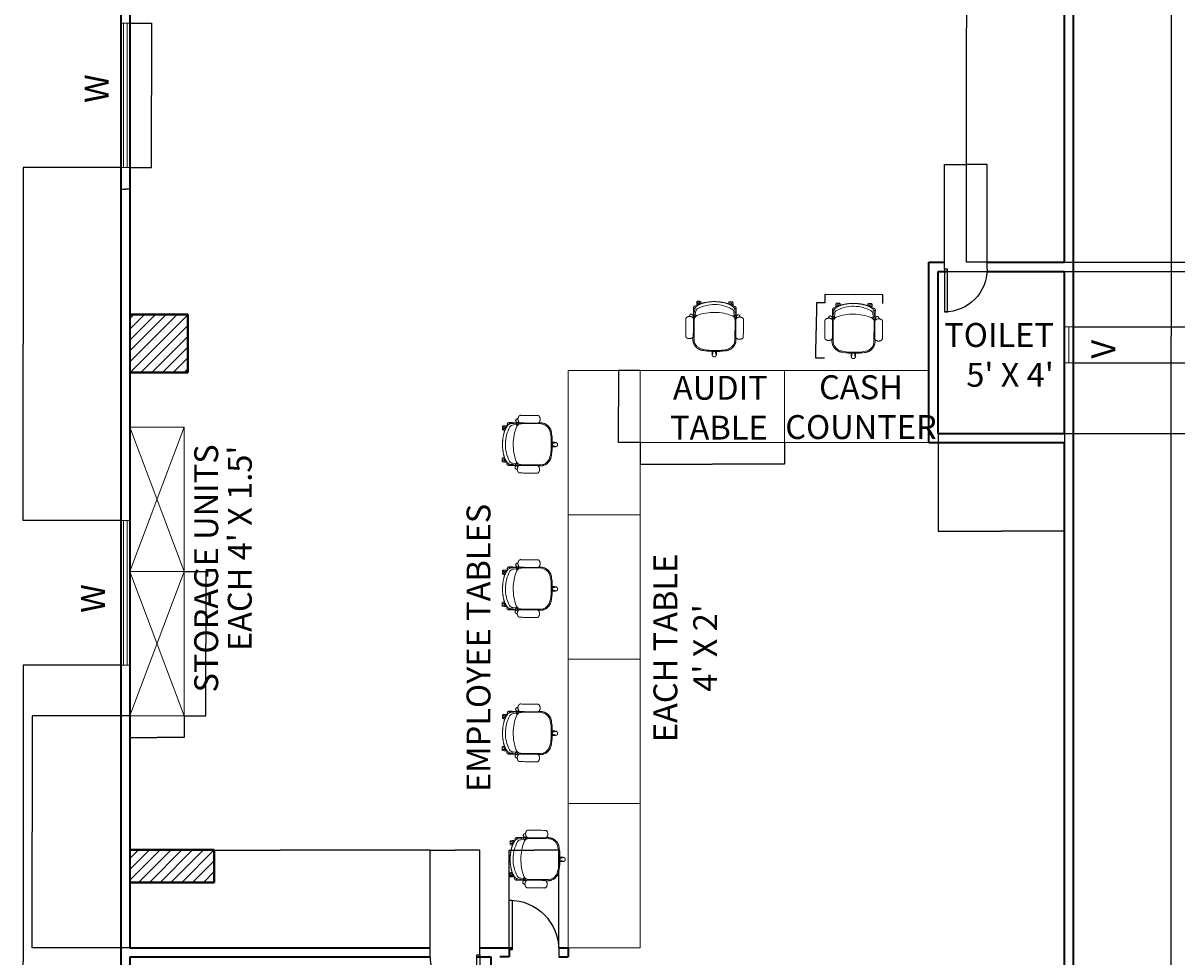
# Model space of a CAD drawing. Units: millimetres. Extents: x -5297 to 19051, y -14478 to 4427.
# Tile 2 of 4: x 1293 to 10888, y -10580 to -2816. Entities that reach past the tile are written whole.
import ezdxf

# ---------------------------------------------------------------- set-up
doc = ezdxf.new("R2010")
doc.units = ezdxf.units.MM
for name, color, linetype, lineweight in [('A-ANNO-DIMS', 2, 'Continuous', 18), ('A-ANNO-TEXT', 7, 'Continuous', 18), ('A-AREA-IDEN', 7, 'Continuous', 25), ('A-COLS', 7, 'Continuous', 40), ('A-COLS-PATT', 252, 'Continuous', 13), ('A-DOOR', 3, 'Continuous', 25), ('A-FLOR-CASE', 9, 'Continuous', 20), ('A-FURN', 8, 'Continuous', 18), ('A-GLAZ', 4, 'Continuous', 18), ('A-WALL', 7, 'Continuous', 35)]:
    doc.layers.add(name, color=color, linetype=linetype, lineweight=lineweight)
doc.styles.get("Standard").update_dxf_attribs({"font": 'arial.ttf'})
doc.dimstyles.get("Standard").update_dxf_attribs({"dimtxt": 0.18, "dimasz": 0.18, "dimexe": 0.18, "dimexo": 0.0625, "dimgap": 0.09, "dimtad": 0, "dimtih": 1, "dimtoh": 1, "dimdec": 4, "dimzin": 0, "dimdsep": 46, "dimtxsty": 'Standard', "dimcen": 0.09, "dimadec": 0, "dimazin": 0, "dimtfac": 1, "dimtdec": 4, "dimtofl": 0, "dimtmove": 0, "dimatfit": 3, "dimfxl": 1, "dimtolj": 1, "dimtzin": 0, "dimarcsym": 0})

# ---------------------------------------------------------------- blocks, each defined once
blk = doc.blocks.new('*U2')
for p, q in [((-700, 0), (-700, -100)), ((0, 0), (0, -100))]:
    blk.add_line(p, q)
blk.add_lwpolyline([(0, 0), (0, 700), (-43.75, 700), (-43.75, 0)], close=True)
blk.add_arc((0, 0), 700, 90, 180)
blk = doc.blocks.new('*U3')
for p, q in [((0, 0), (0, 100)), ((700, 0), (700, 100))]:
    blk.add_line(p, q)
blk.add_lwpolyline([(0, 0), (0, -700), (43.75, -700), (43.75, 0)], close=True)
blk.add_arc((0, 0), 700, 270, 0)
blk = doc.blocks.new('*U4')
for p, q in [((-600, 0), (-600, 100)), ((0, 0), (0, 100))]:
    blk.add_line(p, q)
blk.add_lwpolyline([(0, 0), (0, -600), (-43.75, -600), (-43.75, 0)], close=True)
blk.add_arc((0, 0), 600, 180, 270)
blk = doc.blocks.new('fdss')
at = {"color": 0}
for p, q in [((426, 240), (196, 239)), ((470, 236), (480, 226)), ((480, 225), (479, 223)), ((482, 204), (480, 210)), ((484, 228), (520, 224)), ((617, 196), (646, 196)), ((618, 179), (646, 179)), ((647, 195), (647, 179)), ((426, -240), (196, -239)), ((470, -236), (480, -226)), ((480, -225), (479, -223)), ((482, -204), (480, -210)), ((484, -228), (520, -224)), ((617, -196), (646, -196)), ((618, -179), (646, -179)), ((647, -195), (647, -179))]:
    blk.add_line(p, q, dxfattribs=at)
for points in [[(505, 245), (520, 247), (546, 249), (551, 249)], [(566, 236), (554, 235), (512, 240)], [(33, 21), (34, 20), (36, 19), (37, 18), (37, 18), (39, 18)], [(39, 18), (41, 17), (43, 17), (46, 16), (47, 16), (50, 16), (53, 16), (55, 16), (57, 16), (60, 16), (63, 16)], [(75, -28), (75, 0), (75, 28)], [(33, -21), (34, -20), (36, -19), (37, -18), (37, -18), (39, -18)], [(39, -18), (41, -17), (43, -17), (46, -16), (47, -16), (50, -16), (53, -16), (55, -16), (57, -16), (60, -16), (63, -16)], [(505, -245), (520, -247), (546, -249), (551, -249)], [(566, -236), (554, -235), (512, -240)]]:
    blk.add_lwpolyline(points, dxfattribs=at)
at = {"color": 0, "extrusion": (0, 0, -1)}
for centre, major_axis, start_param, end_param in [((445, 42), (-262, 262), 5.459154, 5.874691), ((201, 128), (-79, 79), 5.969012, 7.027382), ((424, 173), (47, 47), -0.751727, 0.301996), ((424, 175), (54.1, 54.1), -0.544214, -0.156468), ((514, 220), (24.9, 24.9), 3.662908, 4.015109), ((484, 224), (3.3, 3.3), 4.243712, 5.205719), ((484, 229), (-1.47, 1.47), 3.927418, 5.578652), ((-41, 3), (553, 91), -0.204201, 0.167634), ((500, 224), (-12.9, 12.9), 5.819354, 6.506047), ((509, 207), (26.9, 26.9), -1.329065, -0.883773), ((521, 177), (-33.1, 33.1), 0.763307, 1.830683), ((550, 228), (14.8, 14.8), -0.735707, 0.161366), ((545, 180), (-39.3, 39.3), 0.935679, 1.762262), ((193, 0), (-296, 296), 1.856147, 2.355859), ((566, 238), (1.31, 1.31), 0.929037, 2.293349), ((563, 238), (-2.9, 2.9), 1.793197, 2.458506), ((597, 186), (15.6, 15.6), -0.947253, 1.474381), ((621, 198), (-1.12, 1.12), 2.396655, 3.926991), ((621, 177), (-1.12, 1.12), 0.785398, 2.315734), ((646, 195), (0.539, 0.539), -0.785398, 0.785398), ((646, 179), (-0.539, 0.539), 2.356195, 3.926991)]:
    blk.add_ellipse(centre, major_axis=major_axis, ratio=1, start_param=start_param, end_param=end_param, dxfattribs=at)
at = {"color": 0}
for centre, major_axis, start_param, end_param in [((445, -42), (262, 262), 2.317561, 2.733098), ((-41, -3), (-553, 91), 2.937392, 3.309227), ((193, 0), (296, 296), 4.99774, 5.497452), ((201, -128), (79, 79), 2.82742, 3.885789), ((424, -173), (-47, 47), 2.389866, 3.443588), ((424, -175), (-54.1, 54.1), 2.597378, 2.985125), ((514, -220), (-24.9, 24.9), 0.521315, 0.873517), ((484, -224), (-3.3, 3.3), 1.102119, 2.064126), ((484, -229), (1.47, 1.47), 0.785825, 2.437059), ((500, -224), (12.9, 12.9), 2.677762, 3.364454), ((509, -207), (-26.9, 26.9), 1.812527, 2.25782), ((521, -177), (33.1, 33.1), 3.9049, 4.972275), ((550, -228), (-14.8, 14.8), 2.405886, 3.302959), ((545, -180), (39.3, 39.3), 4.077272, 4.903855), ((566, -238), (-1.31, 1.31), 4.07063, 5.434941), ((563, -238), (2.9, 2.9), 4.93479, 5.600098), ((597, -186), (15.6, 15.6), 3.765136, 6.18677), ((621, -177), (1.12, 1.12), 3.926991, 5.457327), ((621, -198), (1.12, 1.12), 5.538248, 7.068583), ((646, -179), (0.539, 0.539), 5.497787, 7.068583), ((646, -195), (-0.539, 0.539), 2.356195, 3.926991)]:
    blk.add_ellipse(centre, major_axis=major_axis, ratio=1, start_param=start_param, end_param=end_param, dxfattribs=at)
for points, weights, knots in [([(436, 337), (338, 337), (240, 337), (234, 338), (228, 335), (217, 328), (212, 315), (204, 293), (212, 271), (217, 258), (228, 251), (234, 248), (240, 248)], [1, 1, 1, 0.962754439438, 1, 0.939418827348, 1, 0.934055427035, 1, 0.939418827348, 1, 0.962754439438, 1], [0, 0, 0, 1, 1, 1.54757, 1.54757, 2.247301, 2.247301, 2.977684, 2.977684, 3.677415, 3.677415, 4.224984, 4.224984, 4.224984]), ([(436, 337), (443, 338), (449, 335), (460, 328), (464, 315), (473, 293), (464, 271), (460, 258), (449, 251), (443, 248), (436, 248), (338, 248), (240, 248)], [1, 0.96275443944, 1, 0.939418827348, 1, 0.934055427035, 1, 0.939418827348, 1, 0.96275443944, 1, 1, 1], [0, 0, 0, 0.54757, 0.54757, 1.247301, 1.247301, 1.977684, 1.977684, 2.677415, 2.677415, 3.224984, 3.224984, 4.224984, 4.224984, 4.224984]), ([(468, 296), (480, 296), (489, 288), (493, 285), (494, 280), (496, 274), (494, 268), (488, 255), (474, 254), (463, 254), (452, 253)], [1, 0.943338632687, 1, 0.968267368414, 1, 0.9394851057, 1, 0.864198855487, 1, 1, 1], [0, 0, 0, 0.676489, 0.676489, 1.181677, 1.181677, 1.881021, 1.881021, 2.935502, 2.935502, 3.935502, 3.935502, 3.935502]), ([(227, 252), (219, 252), (211, 252), (156, 255), (115, 218), (74, 180), (72, 125), (63, 75), (63, 25), (63, 13), (62, 0), (63, -13), (63, -25), (63, -75), (72, -125), (74, -180), (115, -218), (156, -255), (211, -252), (219, -252), (227, -252)], [1, 1, 1, 0.920970329426, 1, 0.920970329426, 1, 0.996764637726, 1, 1, 1, 1, 1, 0.996764637726, 1, 0.920970329426, 1, 0.920970329426, 1, 1, 1], [0, 0, 0, 1, 1, 1.800466, 1.800466, 2.600931, 2.600931, 2.761856, 2.761856, 3.761856, 3.761856, 4.761856, 4.761856, 4.922781, 4.922781, 5.723247, 5.723247, 6.523712, 6.523712, 7.523712, 7.523712, 7.523712]), ([(447, 248), (506, 249), (566, 251), (577, 251), (585, 244), (591, 239), (592, 232), (592, 228), (590, 225), (589, 221), (585, 219)], [1, 1, 1, 0.935512434708, 1, 0.918468104225, 1, 0.965843473499, 1, 0.972653000165, 1], [0, 0, 0, 1, 1, 1.722179, 1.722179, 2.535393, 2.535393, 3.059628, 3.059628, 3.528435, 3.528435, 3.528435]), ([(591, 211), (619, 173), (629, 128), (645, 65), (645, 0), (645, -65), (629, -128), (619, -173), (591, -211)], [1, 0.979760898136, 1, 0.992391068779, 1, 0.992391068779, 1, 0.979760898136, 1], [0, 0, 0, 0.403066, 0.403066, 0.649944, 0.649944, 0.896822, 0.896822, 1.299888, 1.299888, 1.299888]), ([(592, 211), (618, 216), (643, 209), (646, 209), (646, 206), (646, 203), (646, 199), (646, 198), (644, 198), (630, 198), (616, 198)], [1, 0.974666881773, 1, 0.783317345499, 1, 1, 1, 0.707106807826, 1, 1, 1], [0, 0, 0, 0.451139, 0.451139, 1.792762, 1.792762, 2.792762, 2.792762, 4.363559, 4.363559, 5.363559, 5.363559, 5.363559]), ([(618, 177), (631, 177), (644, 177), (645, 177), (645, 176), (646, 176), (646, 175), (646, 172), (646, 168), (646, 166), (643, 165), (631, 161), (619, 161)], [1, 1, 1, 0.923879528314, 1, 0.923879528314, 1, 1, 1, 0.783317456604, 1, 0.992237440768, 1], [0, 0, 0, 1, 1, 1.785398, 1.785398, 2.570796, 2.570796, 3.570796, 3.570796, 4.912419, 4.912419, 5.161781, 5.161781, 5.161781]), ([(33, -20), (22, -27), (10, -20), (-1, -13), (0, 0), (-1, 13), (10, 20), (22, 27), (33, 20)], [1, 0.85579821339, 1, 0.85579821339, 1, 0.855798213391, 1, 0.855798213391, 1], [0, 0, 0, 1.087409, 1.087409, 2.174818, 2.174818, 3.262227, 3.262227, 4.349636, 4.349636, 4.349636]), ([(12, 21), (13, 23), (15, 23), (39, 29), (63, 25)], [1, 0.873023611703, 1, 0.980536821249, 1], [0, 0, 0, 1.018856, 1.018856, 1.414094, 1.414094, 1.414094]), ([(12, -21), (13, -23), (15, -23), (39, -29), (63, -25)], [1, 0.873023611717, 1, 0.980536821249, 1], [0, 0, 0, 1.018856, 1.018856, 1.414094, 1.414094, 1.414094]), ([(464, -271), (460, -258), (449, -251), (443, -248), (436, -248), (338, -248), (240, -248), (234, -248), (228, -251), (217, -258), (212, -271), (204, -293), (212, -315), (217, -328), (228, -335), (234, -338), (240, -337), (338, -337), (436, -337)], [1, 0.939418827349, 1, 0.96275443944, 1, 1, 1, 0.962754439438, 1, 0.939418827349, 1, 0.934055427035, 1, 0.939418827348, 1, 0.962754439438, 1, 1, 1], [0, 0, 0, 0.699731, 0.699731, 1.247301, 1.247301, 2.247301, 2.247301, 2.794871, 2.794871, 3.494602, 3.494602, 4.224984, 4.224984, 4.924715, 4.924715, 5.472285, 5.472285, 6.472285, 6.472285, 6.472285]), ([(447, -248), (506, -249), (566, -251), (577, -251), (585, -244), (591, -239), (592, -232), (592, -228), (590, -225), (589, -221), (585, -219)], [1, 1, 1, 0.935512434708, 1, 0.918468104224, 1, 0.965843473499, 1, 0.972653000166, 1], [0, 0, 0, 1, 1, 1.722179, 1.722179, 2.535393, 2.535393, 3.059628, 3.059628, 3.528435, 3.528435, 3.528435]), ([(468, -296), (480, -296), (489, -288), (493, -285), (494, -280), (496, -274), (494, -268), (488, -255), (474, -254), (463, -254), (452, -253)], [1, 0.943338632687, 1, 0.968267368413, 1, 0.9394851057, 1, 0.864198855486, 1, 1, 1], [0, 0, 0, 0.676489, 0.676489, 1.181677, 1.181677, 1.881021, 1.881021, 2.935502, 2.935502, 3.935502, 3.935502, 3.935502]), ([(592, -211), (618, -216), (643, -209), (646, -209), (646, -206), (646, -203), (646, -199), (646, -198), (644, -198), (630, -198), (616, -198)], [1, 0.974666881774, 1, 0.7833173455, 1, 1, 1, 0.707106807832, 1, 1, 1], [0, 0, 0, 0.451139, 0.451139, 1.792762, 1.792762, 2.792762, 2.792762, 4.363559, 4.363559, 5.363559, 5.363559, 5.363559]), ([(618, -177), (631, -177), (644, -177), (645, -177), (645, -176), (646, -176), (646, -175), (646, -172), (646, -168), (646, -166), (643, -165), (631, -161), (619, -161)], [1, 1, 1, 0.923879528318, 1, 0.923879528318, 1, 1, 1, 0.783317456602, 1, 0.992237440768, 1], [0, 0, 0, 1, 1, 1.785398, 1.785398, 2.570796, 2.570796, 3.570796, 3.570796, 4.912419, 4.912419, 5.161781, 5.161781, 5.161781]), ([(464, -271), (473, -293), (464, -315), (460, -328), (449, -335), (443, -338), (436, -337)], [1, 0.934055427035, 1, 0.939418827348, 1, 0.96275443944, 1], [0, 0, 0, 0.730383, 0.730383, 1.430114, 1.430114, 1.977684, 1.977684, 1.977684])]:
    blk.add_rational_spline(points, weights, degree=2, knots=knots, dxfattribs=at)
blk = doc.blocks.new('TABLE-1200x600')
for p, q in [((0, 0), (0, 1200)), ((0, 1200), (600, 1200)), ((600, 1200), (600, 0)), ((600, 0), (0, 0))]:
    blk.add_line(p, q)
blk = doc.blocks.new('WIN-1200')
for p, q in [((0, 1200.9), (76.2, 1200.9)), ((23.1, 1200.9), (23.1, 0.9)), ((53.1, 1200.9), (53.1, 0.9)), ((0, 0), (76.2, 0))]:
    blk.add_line(p, q)
blk = doc.blocks.new('CABINET-1200x450')
for p, q in [((0, 1200), (450, 1200)), ((0, 0), (0, 1200)), ((450, 1200), (0, 0)), ((450, 0), (0, 1200)), ((450, 1200), (450, 0)), ((450, 0), (0, 0))]:
    blk.add_line(p, q)
blk = doc.blocks.new('*D12')
at = {"layer": 'A-ANNO-DIMS', "color": 0, "lineweight": -2, "transparency": 16777216}
for p, q in [((7962.7, -5142.4), (7963.7, -5070.3)), ((7963.8, -5070.5), (8202.4, -5073.6)), ((8443, -5076.6), (8204.5, -5073.6)), ((8442.3, -5148.5), (8443.2, -5076.5))]:
    blk.add_line(p, q, dxfattribs=at)
at = {"layer": 'A-ANNO-DIMS', "color": 0, "transparency": 16777216}
for points in [[(7963.8, -5070.5), (7963.8, -5070.5), (7963.7, -5070.5)], [(8443, -5076.6), (8443, -5076.7), (8443.2, -5076.6)]]:
    blk.add_solid(points, dxfattribs=at)
at = {"layer": 'Defpoints', "color": 0, "transparency": 16777216}
for p in [(8443.2, -5076.6), (7962.7, -5142.4), (8442.3, -5148.6)]:
    blk.add_point(p, dxfattribs=at)
at = {"layer": 'A-ANNO-DIMS', "color": 0, "transparency": 16777216, "insert": (8203.4, -5073.6), "char_height": 0.18, "attachment_point": 5}
blk.add_mtext('\\A1;CHAIR 480 TYP.', dxfattribs=at)
blk = doc.blocks.new('*D13')
at = {"layer": 'A-ANNO-DIMS', "color": 0, "lineweight": -2, "transparency": 16777216}
for p, q in [((7890.8, -5141.7), (7887.9, -5371.2)), ((7962.7, -5142.4), (7890.6, -5141.5)), ((7884.9, -5601), (7887.9, -5371.5)), ((7956.8, -5602.1), (7884.7, -5601.2))]:
    blk.add_line(p, q, dxfattribs=at)
at = {"layer": 'A-ANNO-DIMS', "color": 0, "transparency": 16777216}
for points in [[(7890.8, -5141.7), (7890.8, -5141.7), (7890.8, -5141.5)], [(7884.9, -5601), (7885, -5601), (7884.9, -5601.2)]]:
    blk.add_solid(points, dxfattribs=at)
at = {"layer": 'Defpoints', "color": 0, "transparency": 16777216}
for p in [(7890.8, -5141.5), (7962.7, -5142.4), (7956.9, -5602.1)]:
    blk.add_point(p, dxfattribs=at)
at = {"layer": 'A-ANNO-DIMS', "color": 0, "transparency": 16777216, "insert": (7887.9, -5371.4), "char_height": 0.18, "attachment_point": 5}
blk.add_mtext('\\A1;460 TYP.', dxfattribs=at)
blk = doc.blocks.new('*D14')
at = {"layer": 'A-ANNO-DIMS', "color": 0, "lineweight": -2, "transparency": 16777216}
for p, q in [((6425, -6303.9), (6425, -6484)), ((7625, -6303.9), (7625, -6484)), ((6425.1, -6483.8), (7023.9, -6483.8)), ((7624.8, -6483.8), (7026.1, -6483.8))]:
    blk.add_line(p, q, dxfattribs=at)
at = {"layer": 'A-ANNO-DIMS', "color": 0, "transparency": 16777216}
for points in [[(6425.1, -6483.8), (6425.1, -6483.8), (6425, -6483.8)], [(7624.8, -6483.8), (7624.8, -6483.8), (7625, -6483.8)]]:
    blk.add_solid(points, dxfattribs=at)
at = {"layer": 'Defpoints', "color": 0, "transparency": 16777216}
for p in [(6425, -6303.8), (7625, -6303.8), (7625, -6483.8)]:
    blk.add_point(p, dxfattribs=at)
at = {"layer": 'A-ANNO-DIMS', "color": 0, "transparency": 16777216, "insert": (7025, -6483.8), "char_height": 0.18, "attachment_point": 5}
blk.add_mtext('\\A1;TABLE 1200 TYP.', dxfattribs=at)
blk = doc.blocks.new('*D15')
at = {"layer": 'A-ANNO-DIMS', "color": 0, "lineweight": -2, "transparency": 16777216}
for p, q in [((6424.9, -5703.8), (6244.8, -5703.8)), ((6245, -5704), (6245, -6003.6)), ((6245, -6303.6), (6245, -6004)), ((6424.9, -6303.8), (6244.8, -6303.8))]:
    blk.add_line(p, q, dxfattribs=at)
at = {"layer": 'A-ANNO-DIMS', "color": 0, "transparency": 16777216}
for points in [[(6244.9, -5704), (6245, -5704), (6245, -5703.8)], [(6244.9, -6303.6), (6245, -6303.6), (6245, -6303.8)]]:
    blk.add_solid(points, dxfattribs=at)
at = {"layer": 'Defpoints', "color": 0, "transparency": 16777216}
for p in [(6425, -5703.8), (6245, -6303.8), (6425, -6303.8)]:
    blk.add_point(p, dxfattribs=at)
at = {"layer": 'A-ANNO-DIMS', "color": 0, "transparency": 16777216, "insert": (6245, -6003.8), "char_height": 0.18, "attachment_point": 5}
blk.add_mtext('\\A1;600 TYP.', dxfattribs=at)
blk = doc.blocks.new('*D16')
at = {"layer": 'A-ANNO-DIMS', "color": 0, "lineweight": -2, "transparency": 16777216}
for p, q in [((2181.8, -2815.9), (2362, -2815.9)), ((2361.8, -2816.1), (2361.8, -3416.2)), ((2361.8, -4016.7), (2361.8, -3416.6)), ((2181.8, -4016.9), (2362, -4016.9))]:
    blk.add_line(p, q, dxfattribs=at)
at = {"layer": 'A-ANNO-DIMS', "color": 0, "transparency": 16777216}
for points in [[(2361.8, -2816.1), (2361.9, -2816.1), (2361.8, -2815.9)], [(2361.8, -4016.7), (2361.9, -4016.7), (2361.8, -4016.9)]]:
    blk.add_solid(points, dxfattribs=at)
at = {"layer": 'Defpoints', "color": 0, "transparency": 16777216}
for p in [(2181.7, -2815.9), (2361.8, -2815.9), (2181.7, -4016.9)]:
    blk.add_point(p, dxfattribs=at)
at = {"layer": 'A-ANNO-DIMS', "color": 0, "transparency": 16777216, "insert": (2361.8, -3416.4), "char_height": 0.18, "attachment_point": 5}
blk.add_mtext('\\A1;WINDOW 1201 TYP.', dxfattribs=at)
blk = doc.blocks.new('*D17')
at = {"layer": 'A-ANNO-DIMS', "color": 0, "lineweight": -2, "transparency": 16777216}
for p, q in [((2105.5, -4016.9), (2105.5, -4197.2)), ((2181.7, -4016.9), (2181.7, -4197.2)), ((2105.7, -4197), (2143.1, -4197)), ((2181.5, -4197), (2144.1, -4197))]:
    blk.add_line(p, q, dxfattribs=at)
at = {"layer": 'A-ANNO-DIMS', "color": 0, "transparency": 16777216}
for points in [[(2105.7, -4197), (2105.7, -4197), (2105.5, -4197)], [(2181.5, -4197), (2181.5, -4197), (2181.7, -4197)]]:
    blk.add_solid(points, dxfattribs=at)
at = {"layer": 'Defpoints', "color": 0, "transparency": 16777216}
for p in [(2105.5, -4016.9), (2181.7, -4016.9), (2181.7, -4197)]:
    blk.add_point(p, dxfattribs=at)
at = {"layer": 'A-ANNO-DIMS', "color": 0, "transparency": 16777216, "insert": (2143.6, -4197), "char_height": 0.18, "attachment_point": 5}
blk.add_mtext('\\A1;76 TYP.', dxfattribs=at)
blk = doc.blocks.new('*D18')
at = {"layer": 'A-ANNO-DIMS', "color": 0, "lineweight": -2, "transparency": 16777216}
for p, q in [((2631.8, -7375.7), (2811.9, -7375.7)), ((2811.7, -7375.9), (2811.7, -7975.5)), ((2811.7, -8575.5), (2811.7, -7975.9)), ((2631.8, -8575.7), (2811.9, -8575.7))]:
    blk.add_line(p, q, dxfattribs=at)
at = {"layer": 'A-ANNO-DIMS', "color": 0, "transparency": 16777216}
for points in [[(2811.7, -7375.9), (2811.7, -7375.9), (2811.7, -7375.7)], [(2811.7, -8575.5), (2811.7, -8575.5), (2811.7, -8575.7)]]:
    blk.add_solid(points, dxfattribs=at)
at = {"layer": 'Defpoints', "color": 0, "transparency": 16777216}
for p in [(2631.7, -7375.7), (2811.7, -7375.7), (2631.7, -8575.7)]:
    blk.add_point(p, dxfattribs=at)
at = {"layer": 'A-ANNO-DIMS', "color": 0, "transparency": 16777216, "insert": (2811.7, -7975.7), "char_height": 0.18, "attachment_point": 5}
blk.add_mtext('\\A1;CABINET 1200 TYP.', dxfattribs=at)
blk = doc.blocks.new('*D19')
at = {"layer": 'A-ANNO-DIMS', "color": 0, "lineweight": -2, "transparency": 16777216}
for p, q in [((2181.7, -8575.7), (2181.7, -8755.9)), ((2631.7, -8575.7), (2631.7, -8755.9)), ((2181.9, -8755.7), (2406.1, -8755.7)), ((2631.5, -8755.7), (2407.3, -8755.7))]:
    blk.add_line(p, q, dxfattribs=at)
at = {"layer": 'A-ANNO-DIMS', "color": 0, "transparency": 16777216}
for points in [[(2181.9, -8755.6), (2181.9, -8755.7), (2181.7, -8755.7)], [(2631.5, -8755.6), (2631.5, -8755.7), (2631.7, -8755.7)]]:
    blk.add_solid(points, dxfattribs=at)
at = {"layer": 'Defpoints', "color": 0, "transparency": 16777216}
for p in [(2181.7, -8575.7), (2631.7, -8575.7), (2631.7, -8755.7)]:
    blk.add_point(p, dxfattribs=at)
at = {"layer": 'A-ANNO-DIMS', "color": 0, "transparency": 16777216, "insert": (2406.7, -8755.7), "char_height": 0.18, "attachment_point": 5}
blk.add_mtext('\\A1;450 TYP.', dxfattribs=at)
blk = doc.blocks.new('*D21')
at = {"layer": 'A-ANNO-DIMS', "color": 0, "lineweight": -2, "transparency": 16777216}
for p, q in [((10028, 2246.2), (10840.6, 2246.2)), ((10840.4, 2246), (10840.4, -5417.6)), ((10840.4, -13081.5), (10840.4, -5417.9)), ((10028, -13081.7), (10840.6, -13081.7))]:
    blk.add_line(p, q, dxfattribs=at)
at = {"layer": 'A-ANNO-DIMS', "color": 0, "transparency": 16777216}
for points in [[(10840.4, 2246), (10840.4, 2246), (10840.4, 2246.2)], [(10840.4, -13081.5), (10840.4, -13081.5), (10840.4, -13081.7)]]:
    blk.add_solid(points, dxfattribs=at)
at = {"layer": 'Defpoints', "color": 0, "transparency": 16777216}
for p in [(10027.9, 2246.2), (10027.9, -13081.7), (10840.4, -13081.7)]:
    blk.add_point(p, dxfattribs=at)
at = {"layer": 'A-ANNO-DIMS', "color": 0, "transparency": 16777216, "insert": (10840.4, -5417.8), "char_height": 0.18, "attachment_point": 5}
blk.add_mtext('\\A1;15328', dxfattribs=at)
blk = doc.blocks.new('*D22')
at = {"layer": 'A-ANNO-DIMS', "color": 0, "lineweight": -2, "transparency": 16777216}
for p, q in [((2105.4, -8153), (1292.8, -8153)), ((1293, -8153.2), (1293, -10616.8)), ((1293, -13080.7), (1293, -10617.1)), ((2105.4, -13080.9), (1292.8, -13080.9))]:
    blk.add_line(p, q, dxfattribs=at)
at = {"layer": 'A-ANNO-DIMS', "color": 0, "transparency": 16777216}
for points in [[(1293, -8153.2), (1293, -8153.2), (1293, -8153)], [(1293, -13080.7), (1293, -13080.7), (1293, -13080.9)]]:
    blk.add_solid(points, dxfattribs=at)
at = {"layer": 'Defpoints', "color": 0, "transparency": 16777216}
for p in [(1293, -8153), (2105.5, -8153), (2105.5, -13080.9)]:
    blk.add_point(p, dxfattribs=at)
at = {"layer": 'A-ANNO-DIMS', "color": 0, "transparency": 16777216, "insert": (1293, -10617), "char_height": 0.18, "attachment_point": 5}
blk.add_mtext('\\A1;4928', dxfattribs=at)
blk = doc.blocks.new('*D23')
at = {"layer": 'A-ANNO-DIMS', "color": 0, "lineweight": -2, "transparency": 16777216}
for p, q in [((2105.4, -4016.9), (1292.8, -4016.9)), ((1293, -4017.1), (1293, -5484.3)), ((1293, -6951.9), (1293, -5484.7)), ((2105.4, -6952.1), (1292.8, -6952.1))]:
    blk.add_line(p, q, dxfattribs=at)
at = {"layer": 'A-ANNO-DIMS', "color": 0, "transparency": 16777216}
for points in [[(1293, -4017.1), (1293, -4017.1), (1293, -4016.9)], [(1293, -6951.9), (1293, -6951.9), (1293, -6952.1)]]:
    blk.add_solid(points, dxfattribs=at)
at = {"layer": 'Defpoints', "color": 0, "transparency": 16777216}
for p in [(1293, -4016.9), (2105.5, -4016.9), (2105.5, -6952.1)]:
    blk.add_point(p, dxfattribs=at)
at = {"layer": 'A-ANNO-DIMS', "color": 0, "transparency": 16777216, "insert": (1293, -5484.5), "char_height": 0.18, "attachment_point": 5}
blk.add_mtext('\\A1;2935', dxfattribs=at)
blk = doc.blocks.new('*D27')
at = {"layer": 'A-ANNO-DIMS', "color": 0, "lineweight": -2, "transparency": 16777216}
for p, q in [((9951.6, -906.2), (9139, -906.2)), ((9139.2, -906.4), (9139.2, -2854.8)), ((9139.2, -4803.6), (9139.2, -2855.2)), ((9951.6, -4803.8), (9139, -4803.8))]:
    blk.add_line(p, q, dxfattribs=at)
at = {"layer": 'A-ANNO-DIMS', "color": 0, "transparency": 16777216}
for points in [[(9139.2, -906.4), (9139.2, -906.4), (9139.2, -906.2)], [(9139.2, -4803.6), (9139.2, -4803.6), (9139.2, -4803.8)]]:
    blk.add_solid(points, dxfattribs=at)
at = {"layer": 'Defpoints', "color": 0, "transparency": 16777216}
for p in [(9139.2, -906.2), (9951.7, -906.2), (9951.7, -4803.8)]:
    blk.add_point(p, dxfattribs=at)
at = {"layer": 'A-ANNO-DIMS', "color": 0, "transparency": 16777216, "insert": (9139.2, -2855), "char_height": 0.18, "attachment_point": 5}
blk.add_mtext('\\A1;3897.6', dxfattribs=at)
blk = doc.blocks.new('*D30')
at = {"layer": 'A-ANNO-DIMS', "color": 0, "lineweight": -2, "transparency": 16777216}
for p, q in [((2181.6, -8575.7), (1369, -8575.7)), ((1369.2, -8575.9), (1369.2, -9539.6)), ((1369.2, -10503.6), (1369.2, -9539.9)), ((2181.6, -10503.8), (1369, -10503.8))]:
    blk.add_line(p, q, dxfattribs=at)
at = {"layer": 'A-ANNO-DIMS', "color": 0, "transparency": 16777216}
for points in [[(1369.2, -8575.9), (1369.2, -8575.9), (1369.2, -8575.7)], [(1369.2, -10503.6), (1369.2, -10503.6), (1369.2, -10503.8)]]:
    blk.add_solid(points, dxfattribs=at)
at = {"layer": 'Defpoints', "color": 0, "transparency": 16777216}
for p in [(1369.2, -8575.7), (2181.7, -8575.7), (2181.7, -10503.8)]:
    blk.add_point(p, dxfattribs=at)
at = {"layer": 'A-ANNO-DIMS', "color": 0, "transparency": 16777216, "insert": (1369.2, -9539.7), "char_height": 0.18, "attachment_point": 5}
blk.add_mtext('\\A1;1928', dxfattribs=at)
blk = doc.blocks.new('*D31')
at = {"layer": 'A-ANNO-DIMS', "color": 0, "lineweight": -2, "transparency": 16777216}
for p, q in [((8901.2, -6227.7), (8901.2, -7040.3)), ((9951.7, -6227.7), (9951.7, -7040.3)), ((8901.3, -7040.1), (9426, -7040.1)), ((9951.5, -7040.1), (9426.9, -7040.1))]:
    blk.add_line(p, q, dxfattribs=at)
at = {"layer": 'A-ANNO-DIMS', "color": 0, "transparency": 16777216}
for points in [[(8901.3, -7040.1), (8901.3, -7040.1), (8901.2, -7040.1)], [(9951.5, -7040.1), (9951.5, -7040.1), (9951.7, -7040.1)]]:
    blk.add_solid(points, dxfattribs=at)
at = {"layer": 'Defpoints', "color": 0, "transparency": 16777216}
for p in [(8901.2, -6227.6), (9951.7, -6227.6), (8901.2, -7040.1)]:
    blk.add_point(p, dxfattribs=at)
at = {"layer": 'A-ANNO-DIMS', "color": 0, "transparency": 16777216, "insert": (9426.4, -7040.1), "char_height": 0.18, "attachment_point": 5}
blk.add_mtext('\\A1;1050.5', dxfattribs=at)
blk = doc.blocks.new('*D32')
at = {"layer": 'A-ANNO-DIMS', "color": 0, "lineweight": -2, "transparency": 16777216}
for p, q in [((8901.2, -4880), (13950.8, -4880)), ((13950.6, -4880.2), (13950.6, -5553.6)), ((13950.6, -6227.4), (13950.6, -5554)), ((8901.2, -6227.6), (13950.8, -6227.6))]:
    blk.add_line(p, q, dxfattribs=at)
at = {"layer": 'A-ANNO-DIMS', "color": 0, "transparency": 16777216}
for points in [[(13950.6, -4880.2), (13950.6, -4880.2), (13950.6, -4880)], [(13950.6, -6227.4), (13950.6, -6227.4), (13950.6, -6227.6)]]:
    blk.add_solid(points, dxfattribs=at)
at = {"layer": 'Defpoints', "color": 0, "transparency": 16777216}
for p in [(8901.2, -4880), (13950.6, -4880), (8901.2, -6227.6)]:
    blk.add_point(p, dxfattribs=at)
at = {"layer": 'A-ANNO-DIMS', "color": 0, "transparency": 16777216, "insert": (13950.6, -5553.8), "char_height": 0.18, "attachment_point": 5}
blk.add_mtext('\\A1;1347.6', dxfattribs=at)
blk = doc.blocks.new('*D35')
at = {"layer": 'A-ANNO-DIMS', "color": 0, "lineweight": -2, "transparency": 16777216}
for p, q in [((8955.2, -4803.7), (8955.2, -3991.1)), ((8955.3, -3991.3), (9131.9, -3991.3)), ((9309.3, -3991.3), (9132.7, -3991.3)), ((9309.5, -4803.7), (9309.5, -3991.1))]:
    blk.add_line(p, q, dxfattribs=at)
at = {"layer": 'A-ANNO-DIMS', "color": 0, "transparency": 16777216}
for points in [[(8955.3, -3991.3), (8955.3, -3991.3), (8955.2, -3991.3)], [(9309.3, -3991.3), (9309.3, -3991.3), (9309.5, -3991.3)]]:
    blk.add_solid(points, dxfattribs=at)
at = {"layer": 'Defpoints', "color": 0, "transparency": 16777216}
for p in [(9309.5, -3991.3), (8955.2, -4803.8), (9309.5, -4803.8)]:
    blk.add_point(p, dxfattribs=at)
at = {"layer": 'A-ANNO-DIMS', "color": 0, "transparency": 16777216, "insert": (9132.3, -3991.3), "char_height": 0.18, "attachment_point": 5}
blk.add_mtext('\\A1;354.3', dxfattribs=at)
blk = doc.blocks.new('*D36')
at = {"layer": 'A-ANNO-DIMS', "color": 0, "lineweight": -2, "transparency": 16777216}
for p, q in [((4678.8, -10503.7), (4678.8, -9691.1)), ((4679, -9691.3), (4885.1, -9691.3)), ((5092, -9691.3), (4885.9, -9691.3)), ((5092.2, -10503.7), (5092.2, -9691.1))]:
    blk.add_line(p, q, dxfattribs=at)
at = {"layer": 'A-ANNO-DIMS', "color": 0, "transparency": 16777216}
for points in [[(4679, -9691.3), (4679, -9691.3), (4678.8, -9691.3)], [(5092, -9691.3), (5092, -9691.3), (5092.2, -9691.3)]]:
    blk.add_solid(points, dxfattribs=at)
at = {"layer": 'Defpoints', "color": 0, "transparency": 16777216}
for p in [(5092.2, -9691.3), (4678.8, -10503.8), (5092.2, -10503.8)]:
    blk.add_point(p, dxfattribs=at)
at = {"layer": 'A-ANNO-DIMS', "color": 0, "transparency": 16777216, "insert": (4885.5, -9691.3), "char_height": 0.18, "attachment_point": 5}
blk.add_mtext('\\A1;413.4', dxfattribs=at)
blk = doc.blocks.new('*D37')
at = {"layer": 'A-ANNO-DIMS', "color": 0, "lineweight": -2, "transparency": 16777216}
for p, q in [((5335.4, -10503.7), (5335.4, -9691.1)), ((5335.6, -9691.3), (5541.7, -9691.3)), ((5748.6, -9691.3), (5542.5, -9691.3)), ((5748.8, -10503.7), (5748.8, -9691.1))]:
    blk.add_line(p, q, dxfattribs=at)
at = {"layer": 'A-ANNO-DIMS', "color": 0, "transparency": 16777216}
for points in [[(5335.6, -9691.3), (5335.6, -9691.3), (5335.4, -9691.3)], [(5748.6, -9691.3), (5748.6, -9691.3), (5748.8, -9691.3)]]:
    blk.add_solid(points, dxfattribs=at)
at = {"layer": 'Defpoints', "color": 0, "transparency": 16777216}
for p in [(5748.8, -9691.3), (5335.4, -10503.8), (5748.8, -10503.8)]:
    blk.add_point(p, dxfattribs=at)
at = {"layer": 'A-ANNO-DIMS', "color": 0, "transparency": 16777216, "insert": (5542.1, -9691.3), "char_height": 0.18, "attachment_point": 5}
blk.add_mtext('\\A1;413.4', dxfattribs=at)
blk = doc.blocks.new('*D38')
at = {"layer": 'A-ANNO-DIMS', "color": 0, "lineweight": -2, "transparency": 16777216}
for p, q in [((2181.7, -10503.7), (2181.7, -9691.1)), ((2181.9, -9691.3), (3429.9, -9691.3)), ((4678.7, -9691.3), (3430.6, -9691.3)), ((4678.8, -10503.7), (4678.8, -9691.1))]:
    blk.add_line(p, q, dxfattribs=at)
at = {"layer": 'A-ANNO-DIMS', "color": 0, "transparency": 16777216}
for points in [[(2181.9, -9691.3), (2181.9, -9691.3), (2181.7, -9691.3)], [(4678.7, -9691.3), (4678.7, -9691.3), (4678.8, -9691.3)]]:
    blk.add_solid(points, dxfattribs=at)
at = {"layer": 'Defpoints', "color": 0, "transparency": 16777216}
for p in [(4678.8, -9691.3), (2181.7, -10503.8), (4678.8, -10503.8)]:
    blk.add_point(p, dxfattribs=at)
at = {"layer": 'A-ANNO-DIMS', "color": 0, "transparency": 16777216, "insert": (3430.3, -9691.3), "char_height": 0.18, "attachment_point": 5}
blk.add_mtext('\\A1;2497', dxfattribs=at)
blk = doc.blocks.new('*D41')
at = {"layer": 'A-ANNO-DIMS', "color": 0, "lineweight": -2, "transparency": 16777216}
for p, q in [((10028, -5340.2), (13950.8, -5340.2)), ((13950.6, -5340.4), (13950.6, -5490.1)), ((13950.6, -5640.1), (13950.6, -5490.4)), ((10028, -5640.2), (13950.8, -5640.2))]:
    blk.add_line(p, q, dxfattribs=at)
at = {"layer": 'A-ANNO-DIMS', "color": 0, "transparency": 16777216}
for points in [[(13950.6, -5340.4), (13950.6, -5340.4), (13950.6, -5340.2)], [(13950.6, -5640.1), (13950.6, -5640.1), (13950.6, -5640.2)]]:
    blk.add_solid(points, dxfattribs=at)
at = {"layer": 'Defpoints', "color": 0, "transparency": 16777216}
for p in [(10027.9, -5340.2), (10027.9, -5640.2), (13950.6, -5640.2)]:
    blk.add_point(p, dxfattribs=at)
at = {"layer": 'A-ANNO-DIMS', "color": 0, "transparency": 16777216, "insert": (13950.6, -5490.2), "char_height": 0.18, "attachment_point": 5}
blk.add_mtext('\\A1;300', dxfattribs=at)
blk = doc.blocks.new('*D42')
at = {"layer": 'A-ANNO-DIMS', "color": 0, "lineweight": -2, "transparency": 16777216}
for p, q in [((9951.8, -4803.8), (13950.8, -4803.8)), ((13950.6, -4804), (13950.6, -5071.8)), ((13950.6, -5340.1), (13950.6, -5072.2)), ((10028, -5340.2), (13950.8, -5340.2))]:
    blk.add_line(p, q, dxfattribs=at)
at = {"layer": 'A-ANNO-DIMS', "color": 0, "transparency": 16777216}
for points in [[(13950.6, -4804), (13950.6, -4804), (13950.6, -4803.8)], [(13950.6, -5340.1), (13950.6, -5340.1), (13950.6, -5340.2)]]:
    blk.add_solid(points, dxfattribs=at)
at = {"layer": 'Defpoints', "color": 0, "transparency": 16777216}
for p in [(9951.7, -4803.8), (10027.9, -5340.2), (13950.6, -5340.2)]:
    blk.add_point(p, dxfattribs=at)
at = {"layer": 'A-ANNO-DIMS', "color": 0, "transparency": 16777216, "insert": (13950.6, -5072), "char_height": 0.18, "attachment_point": 5}
blk.add_mtext('\\A1;536.4', dxfattribs=at)

msp = doc.modelspace()

# ---------------------------------------------------------------- hatches: boundary and pattern name
at = {"layer": 'A-COLS-PATT'}
h = msp.add_hatch(dxfattribs=at)
h.set_pattern_fill('ANSI31', color=256, scale=20)
h.paths.add_polyline_path([(2881.7, 2169.99), (2181.7, 2169.99), (2181.7, 1689.99), (2781.7, 1689.99), (2881.7, 1689.99)])
h.paths.add_polyline_path([(9951.7, 2169.99), (9731.7, 2169.99), (9731.7, 1689.99), (9951.7, 1689.99)])
h.paths.add_polyline_path([(2651.7, -1930.01), (2181.7, -1930.01), (2181.7, -2200.01), (2651.7, -2200.01)])
h.paths.add_polyline_path([(2661.7, -5240.01), (2181.7, -5240.01), (2181.7, -5720.01), (2661.7, -5720.01)])
h.paths.add_polyline_path([(2881.7, -9690.01), (2181.7, -9690.01), (2181.7, -9960.01), (2881.7, -9960.01)])

# ---------------------------------------------------------------- linework, layer by layer
at = {"layer": 'A-COLS'}
for p, q in [((2181.7, -5240.01), (2661.7, -5240.01)), ((2661.7, -5240.01), (2661.7, -5720.01)), ((2661.7, -5720.01), (2181.7, -5720.01)), ((2181.7, -9690.01), (2881.7, -9690.01)), ((2881.7, -9690.01), (2881.7, -9960.01)), ((2881.7, -9960.01), (2181.7, -9960.01))]:
    msp.add_line(p, q, dxfattribs=at)
at = {"layer": 'A-GLAZ'}
for p, q in [((9951.7, -5340.23), (10027.9, -5340.23)), ((9989.8, -5340.23), (9989.8, -5640.23)), ((9989.8, -5640.23), (9951.7, -5640.23)), ((9989.8, -5640.23), (10027.9, -5640.23))]:
    msp.add_line(p, q, dxfattribs=at)
at = {"layer": 'A-WALL'}
for p, q in [((2105.5, 2246.19), (2105.5, -13080.86)), ((10027.9, -13081.69), (10027.9, 2246.19)), ((2181.7, 2169.99), (2181.7, -10503.81)), ((9951.7, -4803.81), (9951.7, -906.21)), ((8824.97, -6303.81), (8824.97, -4803.81)), ((8824.97, -4803.81), (8955.17, -4803.81)), ((8901.17, -6227.61), (8901.17, -4880.01)), ((8901.17, -4880.01), (8981, -4880.01)), ((9309.07, -4880.01), (9951.7, -4880.01)), ((9309.49, -4803.81), (9951.7, -4803.81)), ((9951.7, -6227.61), (9951.7, -4880.01)), ((8901.17, -6227.61), (9951.7, -6227.61)), ((8824.97, -6303.81), (9951.7, -6303.81)), ((9951.7, -12980.01), (9951.7, -6303.81)), ((2181.7, -10503.81), (4678.84, -10503.81)), ((5092.22, -10503.81), (5257.9, -10503.81)), ((5257.9, -10503.81), (5334.1, -10503.81)), ((5334.1, -10503.81), (5334.1, -10580.01)), ((5335.39, -10503.81), (5359.94, -10503.81)), ((5747.12, -10503.81), (5748.77, -10503.81)), ((5748.77, -10503.81), (5824.97, -10503.81)), ((5824.97, -10503.81), (5824.97, -10580.01)), ((2181.7, -10580.01), (4679.2, -10580.01)), ((2181.7, -10580.01), (2181.7, -12980.01)), ((5066.38, -10580.01), (5181.7, -10580.01)), ((5181.7, -10580.01), (5181.7, -12980.01)), ((5334.1, -10580.01), (5257.9, -10580.01)), ((5747.48, -10580.01), (5824.97, -10580.01))]:
    msp.add_line(p, q, dxfattribs=at)

# ---------------------------------------------------------------- block references
at = {"layer": 'A-DOOR', "xscale": -0.5905371076916341, "yscale": 0.5905371076916341, "zscale": 0.5905371076916341}
msp.add_blockref('*U4', (8955.17, -4862.86), dxfattribs=at)
at = {"layer": 'A-DOOR', "xscale": -0.5905371076916341, "yscale": 0.5905371076916341, "zscale": 0.5905371076916341, "rotation": 180}
for name, p in [('*U3', (5334.1, -10520.96)), ('*U2', (5092.22, -10562.86))]:
    msp.add_blockref(name, p, dxfattribs=at)
at = {"layer": 'A-FLOR-CASE'}
for p in [(2181.7, -7375.67), (2181.7, -8575.67)]:
    msp.add_blockref('CABINET-1200x450', p, dxfattribs=at)
at = {"layer": 'A-FURN', "xscale": -0.7108527329127514, "yscale": 0.7108527329127514, "zscale": 0.7108527329127514}
for p, rotation in [((7040.1, -5590.35), 269.2672508438734), ((8196.63, -5605.16), 269.2672508438734), ((5738.06, -6320.7), 359.2672508438734), ((5738.06, -7520.7), 359.2672508438734), ((5738.06, -8720.7), 359.2672508438734), ((5801.72, -9769.5), 359.2672508438734)]:
    msp.add_blockref('fdss', p, dxfattribs=dict(at, rotation=rotation))
at = {"layer": 'A-FURN'}
for p in [(5824.97, -6903.81), (5824.97, -8103.81), (5824.97, -9303.81), (5824.97, -10503.81)]:
    msp.add_blockref('TABLE-1200x600', p, dxfattribs=at)
at = {"layer": 'A-FURN', "rotation": 270.0000000000002}
for p in [(6424.97, -5703.81), (7624.97, -5703.81)]:
    msp.add_blockref('TABLE-1200x600', p, dxfattribs=at)
at = {"layer": 'A-GLAZ'}
for p in [(2105.5, -4016.87), (2105.5, -8153.04)]:
    msp.add_blockref('WIN-1200', p, dxfattribs=at)

# ---------------------------------------------------------------- texts
at = {"layer": 'A-ANNO-TEXT', "char_height": 198.615, "attachment_point": 3, "rotation": 90}
for s, insert in [('\\pxqc;{\\fArial|b1|i0|c0|p34;W}', (1805.02, -1961)), ('\\pxqc;{\\fArial|b1|i0|c0|p34;V}', (10176.34, -4127.65)), ('\\pxqc;{\\fArial|b1|i0|c0|p34;STORAGE UNITS}', (2716.23, -5950.25)), ("\\pxqc;{\\fArial|b1|i0|c0|p34;EACH 4' X 1.5'}", (2995.59, -5783.02)), ('\\pxqc;{\\fArial|b1|i0|c0|p34;EMPLOYEE TABLES}', (4980.62, -6611.2)), ("\\pxqc;{\\fArial|b1|i0|c0|p34;EACH TABLE ^J4' X 2'}", (6534.81, -6611.2)), ('\\pxqc;{\\fArial|b1|i0|c0|p34;W}', (1774.6, -6200.26))]:
    msp.add_mtext_dynamic_manual_height_columns(s, width=2799.8532, gutter_width=413.78, heights=[0], dxfattribs=dict(at, insert=insert))
at = {"layer": 'A-ANNO-TEXT', "char_height": 198.615, "attachment_point": 3}
for s, width, insert in [('{\\fArial|b1|i0|c0|p34;AUDIT \\PTABLE}', 840.8417, (7484.74, -5748.93)), ('\\pxqc;{\\fArial|b1|i0|c0|p34;CASH^JCOUNTER}', 1401.5231, (8961.04, -5744.35))]:
    msp.add_mtext_dynamic_manual_height_columns(s, width=width, gutter_width=413.78, heights=[0], dxfattribs=dict(at, insert=insert))
at = {"layer": 'A-AREA-IDEN', "insert": (9864.43, -5309.8), "char_height": 198.615, "attachment_point": 3}
msp.add_mtext_dynamic_manual_height_columns("{\\fArial|b1|i0|c0|p34;TOILET^J5' X 4'}", width=840.8417, gutter_width=413.78, heights=[0], dxfattribs=at)

# ---------------------------------------------------------------- dimensions: what is measured, and where the dimension line sits
at = {"layer": 'A-ANNO-DIMS'}
for base, p1, p2, angle, override, picture, middle in [((10840.4, -13081.69), (10027.9, 2246.19), (10027.9, -13081.69), 270, {"dimdec": 0, "dimlfac": 1, "dimrnd": 0, "dimzin": 0, "dimdsep": 46, "dimlunit": 2}, '*D21', (10840.4, -5417.75)), ((9139.2, -906.21), (9951.7, -4803.81), (9951.7, -906.21), 90, {"dimdec": 1, "dimlfac": 1, "dimrnd": 0, "dimzin": 0, "dimdsep": 46, "dimlunit": 2}, '*D27', (9139.2, -2855.01)), ((1293, -4016.87), (2105.5, -6952.11), (2105.5, -4016.87), 90, {"dimdec": 0, "dimlfac": 1, "dimrnd": 0, "dimzin": 0, "dimdsep": 46, "dimlunit": 2}, '*D23', (1293, -5484.49)), ((13950.61, -4880.01), (8901.17, -6227.61), (8901.17, -4880.01), 90, {"dimdec": 1, "dimlfac": 1, "dimrnd": 0, "dimzin": 0, "dimdsep": 46, "dimlunit": 2}, '*D32', (13950.61, -5553.81)), ((13950.61, -5340.23), (9951.7, -4803.81), (10027.9, -5340.23), 90, {"dimdec": 1, "dimlfac": 1, "dimrnd": 0, "dimzin": 0, "dimdsep": 46, "dimlunit": 2}, '*D42', (13950.61, -5072.02)), ((13950.61, -5640.23), (10027.9, -5340.23), (10027.9, -5640.23), 90, {"dimdec": 0, "dimlfac": 1, "dimrnd": 0, "dimzin": 0, "dimdsep": 46, "dimlunit": 2}, '*D41', (13950.61, -5490.23)), ((8901.17, -7040.11), (9951.7, -6227.61), (8901.17, -6227.61), 180, {"dimdec": 1, "dimlfac": 1, "dimrnd": 0, "dimzin": 0, "dimdsep": 46, "dimlunit": 2}, '*D31', (9426.44, -7040.11)), ((1293, -8153.04), (2105.5, -13080.86), (2105.5, -8153.04), 90, {"dimdec": 0, "dimlfac": 1, "dimrnd": 0, "dimzin": 0, "dimdsep": 46, "dimlunit": 2}, '*D22', (1293, -10616.95)), ((1369.2, -8575.67), (2181.7, -10503.81), (2181.7, -8575.67), 90, {"dimdec": 0, "dimlfac": 1, "dimrnd": 0, "dimzin": 0, "dimdsep": 46, "dimlunit": 2}, '*D30', (1369.2, -9539.74))]:
    dim = msp.add_linear_dim(base=base, p1=p1, p2=p2, angle=angle, dimstyle='Standard', override=override, dxfattribs=at)
    dim.commit()
    dim.dimension.update_dxf_attribs({"geometry": picture, "text_midpoint": middle})
for base, p1, p2, angle, text, picture, middle in [((2361.84, -2815.94), (2181.7, -4016.87), (2181.7, -2815.94), 90, 'WINDOW <> TYP.', '*D16', (2361.84, -3416.41)), ((8443.21, -5076.63), (7962.74, -5142.43), (8442.29, -5148.56), 359.267251, 'CHAIR <> TYP.', '*D12', (8203.44, -5073.56)), ((7890.81, -5141.51), (7956.86, -5602.14), (7962.74, -5142.43), 89.267251, '<> TYP.', '*D13', (7887.87, -5371.36)), ((6244.97, -6303.81), (6424.97, -5703.81), (6424.97, -6303.81), 270, '<> TYP.', '*D15', (6244.97, -6003.81)), ((7624.97, -6483.81), (6424.97, -6303.81), (7624.97, -6303.81), 0, 'TABLE <> TYP.', '*D14', (7024.97, -6483.81)), ((2811.7, -7375.67), (2631.7, -8575.67), (2631.7, -7375.67), 90, 'CABINET <> TYP.', '*D18', (2811.7, -7975.67))]:
    dim = msp.add_linear_dim(base=base, p1=p1, p2=p2, angle=angle, text=text, dimstyle='Standard', override={"dimdec": 0, "dimlfac": 1, "dimrnd": 0, "dimzin": 0, "dimdsep": 46, "dimlunit": 2}, dxfattribs=at)
    dim.commit()
    dim.dimension.update_dxf_attribs({"geometry": picture, "text_midpoint": middle})
for base, p1, p2, picture, middle in [((2181.7, -4197.01), (2105.5, -4016.87), (2181.7, -4016.87), '*D17', (2143.6, -4197.01)), ((2631.7, -8755.67), (2181.7, -8575.67), (2631.7, -8575.67), '*D19', (2406.7, -8755.67))]:
    dim = msp.add_linear_dim(base=base, p1=p1, p2=p2, text='<> TYP.', dimstyle='Standard', override={"dimdec": 0, "dimlfac": 1, "dimrnd": 0, "dimzin": 0, "dimdsep": 46, "dimlunit": 2}, dxfattribs=at)
    dim.commit()
    dim.dimension.update_dxf_attribs({"geometry": picture, "text_midpoint": middle})
for base, p1, p2, override, picture, middle in [((9309.49, -3991.31), (8955.17, -4803.81), (9309.49, -4803.81), {"dimdec": 1, "dimlfac": 1, "dimrnd": 0, "dimzin": 0, "dimdsep": 46, "dimlunit": 2}, '*D35', (9132.33, -3991.31)), ((4678.84, -9691.31), (2181.7, -10503.81), (4678.84, -10503.81), {"dimdec": 0, "dimlfac": 1, "dimrnd": 0, "dimzin": 0, "dimdsep": 46, "dimlunit": 2}, '*D38', (3430.27, -9691.31)), ((5092.22, -9691.31), (4678.84, -10503.81), (5092.22, -10503.81), {"dimdec": 1, "dimlfac": 1, "dimrnd": 0, "dimzin": 0, "dimdsep": 46, "dimlunit": 2}, '*D36', (4885.53, -9691.31)), ((5748.77, -9691.31), (5335.39, -10503.81), (5748.77, -10503.81), {"dimdec": 1, "dimlfac": 1, "dimrnd": 0, "dimzin": 0, "dimdsep": 46, "dimlunit": 2}, '*D37', (5542.08, -9691.31))]:
    dim = msp.add_linear_dim(base=base, p1=p1, p2=p2, dimstyle='Standard', override=override, dxfattribs=at)
    dim.commit()
    dim.dimension.update_dxf_attribs({"geometry": picture, "text_midpoint": middle})

doc.saveas('drawing.dxf')
